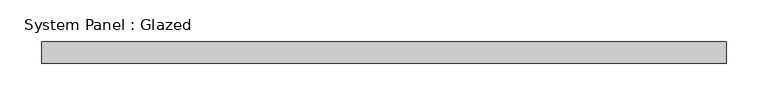
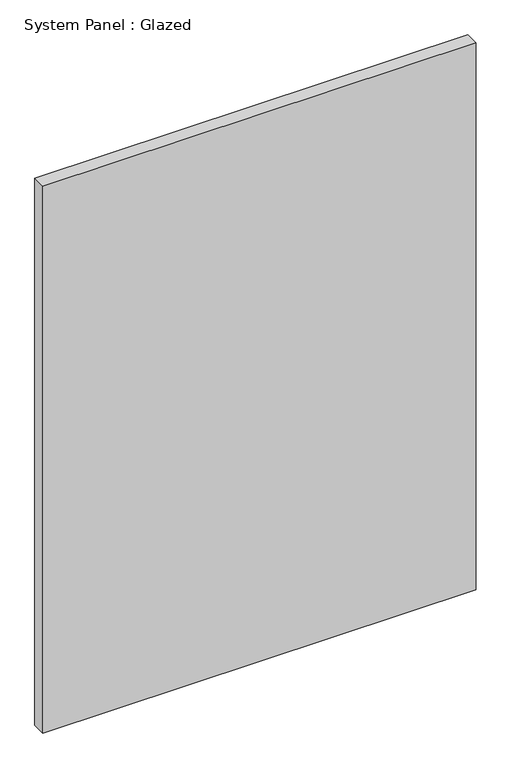
"""IFC4 building model written with IfcOpenShell, lengths in millimetres: plate geometry, System Panel : Glazed."""

from ifc_helpers import new_model, si_unit, origin, origin_with_axes, place, context, project, spatial, polyline, outline, extrude, source, transform, mapped, element, save


def system_panel_glazed_25f99c47(model_context):
    return source(origin(), model_context, "Body", "SweptSolid", [
        extrude(outline(polyline([(409.4264909, -44.45), (-409.4264909, -44.45), (-409.4264909, -19.05), (409.4264909, -19.05), (409.4264909, -44.45)])), origin_with_axes(), (0.0, 0.0, 1.0), 1092.2),
    ])


if __name__ == "__main__":
    model = new_model("IFC4")
    model_context = context("Model", 3, world=origin())
    ifc_project = project(units=[si_unit("LENGTHUNIT", "METRE", prefix="MILLI")], contexts=[model_context])
    site = spatial("IfcSite", under=ifc_project)
    building = spatial("IfcBuilding", under=site)
    placement = place(None, origin())
    system_panel_glazed_shape = system_panel_glazed_25f99c47(model_context)
    element("IfcPlate", 1, ObjectType="System Panel : Glazed", at=placement, inside=building, context=model_context, shape_type="MappedRepresentation", body=[
        mapped(system_panel_glazed_shape, transform((0.0, 0.0, 0.0), x_axis=(1.0, 0.0, 0.0), y_axis=(0.0, 1.0, 0.0), z_axis=(0.0, 0.0, 1.0))),
    ])
    save(model, "model.ifc")

# Revit data of these elements
# Type "System Panel : Glazed"
#   Construction Type Id = "GSP4R"
#   Analytic Construction = "1/8 in Pilkington single glazing"
#   Visual Light Transmittance = 0.9
#   Solar Heat Gain Coefficient = 0.86
#   Heat Transfer Coefficient (U) = 1.18115 BTU/(h·ft²·°F)
#   Define Thermal Properties by = 1
# Element 1 (IfcPlate, "System Panel : Glazed")
#   Materials on its faces: "Glass"
# Materials
#   "Glass": class "Glass", colour RGB 0 128 192, transparency 0.75, Description = "Soda Lime Glass", Cost = 0
